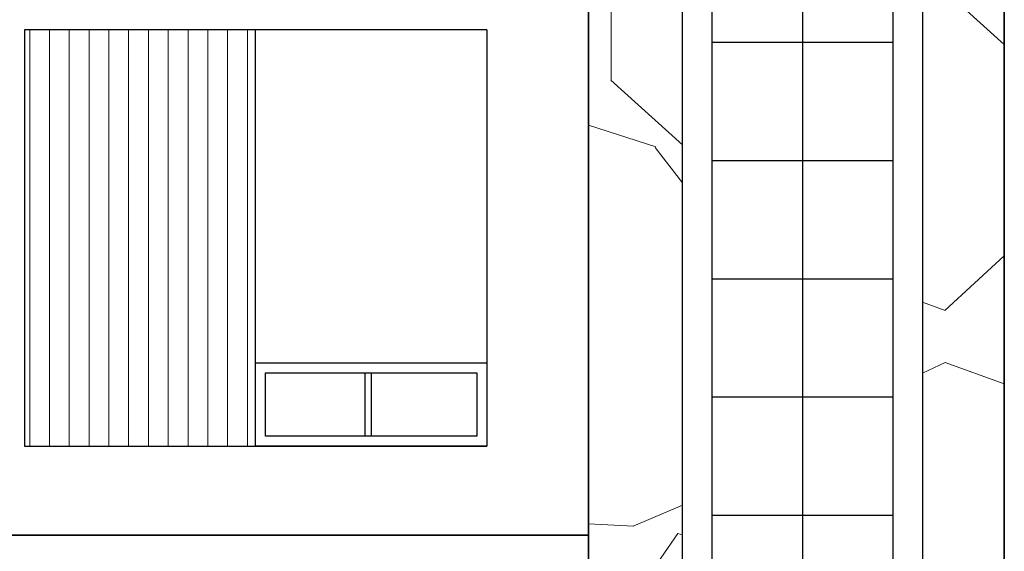
# Model space of a CAD drawing. Units: inches. Extents: x 3 to 303, y 4 to 326.
# Tile 5 of 6: x 104 to 303, y 120 to 228. Entities that reach past the tile are written whole.
import ezdxf

# ---------------------------------------------------------------- set-up
doc = ezdxf.new("R2010")
doc.units = ezdxf.units.IN
doc.header["$MEASUREMENT"] = 0
for name, color, linetype, lineweight in [('A-ELEV', 7, 'Continuous', 35), ('A-ELEV-PATT', 8, 'Continuous', 13), ('A-GLAZ', 4, 'Continuous', 25)]:
    doc.layers.add(name, color=color, linetype=linetype, lineweight=lineweight)

msp = doc.modelspace()

# ---------------------------------------------------------------- hatches: boundary and pattern name
at = {"layer": 'A-ELEV-PATT'}
h = msp.add_hatch(dxfattribs=at)
h.set_pattern_fill('GRAVEL', color=256, scale=150, angle=90)
h.set_pattern_definition([(318.0128, (-159.712, 82.498), (1350, -1200), [20.18, -1997.863]), (274.9697, (-144.712, 68.998), (-150, 1800), [34.63, -3428.3887]), (222.5104, (-141.712, 34.498), (1650, 1500), [24.418, -2417.405]), (357.2737, (-104.212, -24.002), (-3000, 150), [31.536, -3122.034]), (22.8337, (-72.712, -25.502), (-1800, -750), [30.923, -3061.406]), (87.2737, (-44.212, -13.502), (-150, -3000), [31.536, -3122.034]), (127.6942, (-42.712, 17.9977), (1500, -1950), [41.7043, -4128.7273]), (162.2553, (-68.212, 50.998), (-3300, 1050), [39.373, -3897.948]), (211.4296, (-105.712, 62.998), (-1950, -1200), [31.6425, -3132.611]), (265.2364, (-132.712, 46.498), (150, 1650), [36.125, -1770.114]), (312.3974, (-135.712, 10.4977), (1650, -1800), [46.717, -4625.0063]), (228.814, (-102.712, 124.498), (-900, -1050), [15.945, -1578.577]), (261.4692, (-113.212, 112.498), (300, 1950), [30.3356, -3003.227]), (315, (-117.71, 82.5), (150, -3e-14), [21.213, -190.92]), (293.1986, (-135.712, 71.998), (-300, 750), [11.424, -1130.942]), (21.8014, (-131.212, 61.498), (-450, -150), [16.155, -791.62]), (120.964, (-116.212, 67.498), (-300, 450), [26.24, -848.403]), (251.565, (-129.71, 90), (150, 300), [18.974, -455.368]), (106.3895, (-131.212, -25.502), (-450, 1500), [26.58, -2631.427]), (160.3462, (-138.712, -0.002), (1650, -600), [22.299, -2207.611]), (23.1986, (-159.712, 89.998), (-750, -300), [22.847, -1119.519]), (73.6105, (-138.712, 98.998), (-450, -1500), [26.58, -2631.427]), (69.444, (-38.212, -25.502), (-300, -750), [25.632, -1255.969]), (24.7751, (-29.212, -1.502), (-1650, -750), [21.477, -2126.1965]), (156.8014, (-9.712, 91.498), (-750, 300), [22.847, -1119.519]), (107.354, (-30.712, 100.498), (600, -1950), [25.145, -2489.3135]), (159.444, (-9.712, 17.998), (750, -300), [12.816, -1268.785]), (191.31, (-9.712, 82.498), (-600, -150), [7.649, -757.204]), (255.964, (-17.21, 80.998), (150, 450), [30.923, -587.543]), (276.009, (-24.712, 50.998), (-150, 1500), [28.6575, -2837.0885]), (33.69, (-102.71, 67.498), (-300, -150), [21.633, -519.2]), (83.1572, (-84.712, 79.498), (300, 2550), [37.769, -3739.1344]), (150.9454, (-80.212, 116.998), (1050, -600), [15.443, -1528.901]), (180, (-93.71, 124.5), (-150, -150), [9, -141]), (210.2564, (-29.212, 47.998), (1050, 600), [20.839, -2063.028]), (138.0128, (-47.212, 37.498), (-1350, 1200), [40.361, -1977.683]), (90, (-77.21, 64.5), (-150, 150), [39, -111]), (55.3048, (-77.212, 103.498), (1050, 1500), [23.717, -2347.991]), (344.0546, (-63.712, 122.998), (600, -150), [21.84, -1070.176]), (297.646, (-42.712, 116.998), (1500, -2850), [35.56, -3520.421]), (265.426, (-26.212, 85.498), (-150, -1950), [37.62, -3724.361])])
h.paths.add_polyline_path([(303.23, 123.62), (303.23, 243.62), (303.23, 325.61), (219.23, 325.61), (219.23, 243.62), (219.23, 63.62), (232.73, 63.62), (232.73, 80.06), (244.07, 80.06), (244.07, 63.62), (257.57, 63.62), (257.57, 80.06), (268.91, 80.06), (268.91, 63.62), (282.42, 63.62), (282.42, 80.06), (293.76, 80.06), (293.76, 63.62), (303.23, 63.62)])
h.paths.add_polyline_path([(286.72, 105.38), (238.22, 105.38), (238.22, 300.66), (286.72, 300.66)], flags=16)
h.paths.add_polyline_path([(280.72, 111.38), (244.22, 111.38), (244.22, 294.66), (280.72, 294.66)], flags=0)
h = msp.add_hatch(dxfattribs=at)
h.set_pattern_fill('_USER', color=256, scale=4, angle=90, pattern_type=0)
h.set_pattern_definition([(90, (-9.712, -25.5023), (-4, 2e-16), [])])
h.paths.add_polyline_path([(151.94, 225.62), (105.23, 225.62), (105.23, 141.62), (151.94, 141.62)])

# ---------------------------------------------------------------- linework, layer by layer
at = {"layer": 'A-ELEV'}
for p, q in [((219.23, 3.62), (219.23, 243.62)), ((303.23, 123.62), (303.23, 243.62)), ((219.23, 123.62), (15.23, 123.62)), ((15.23, 123.62), (219.23, 123.62)), ((303.23, 3.62), (303.23, 123.62))]:
    msp.add_line(p, q, dxfattribs=at)
at = {"layer": 'A-GLAZ'}
for p, q in [((262.47, 294.66), (262.47, 111.38)), ((105.23, 225.62), (105.23, 141.62)), ((198.65, 225.62), (105.23, 225.62)), ((151.94, 141.62), (151.94, 225.62)), ((198.65, 225.62), (198.65, 141.62)), ((244.22, 223.11), (280.72, 223.11)), ((244.22, 199.26), (280.72, 199.26)), ((244.22, 175.41), (280.72, 175.41)), ((244.22, 151.56), (280.72, 151.56)), ((105.23, 141.62), (198.65, 141.62)), ((244.22, 127.71), (280.72, 127.71))]:
    msp.add_line(p, q, dxfattribs=at)
for points in [[(238.22, 300.66), (286.72, 300.66), (286.72, 105.38), (238.22, 105.38)], [(244.22, 294.66), (280.72, 294.66), (280.72, 111.38), (244.22, 111.38)], [(151.94, 158.4), (198.65, 158.4), (198.65, 141.62), (151.94, 141.62)], [(153.94, 156.4), (196.65, 156.4), (196.65, 143.62), (153.94, 143.62)], [(174.08, 156.4), (175.29, 156.4), (175.29, 143.62), (174.08, 143.62)]]:
    msp.add_lwpolyline(points, close=True, dxfattribs=at)

doc.saveas('drawing.dxf')
